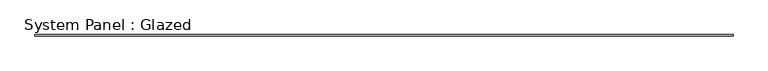
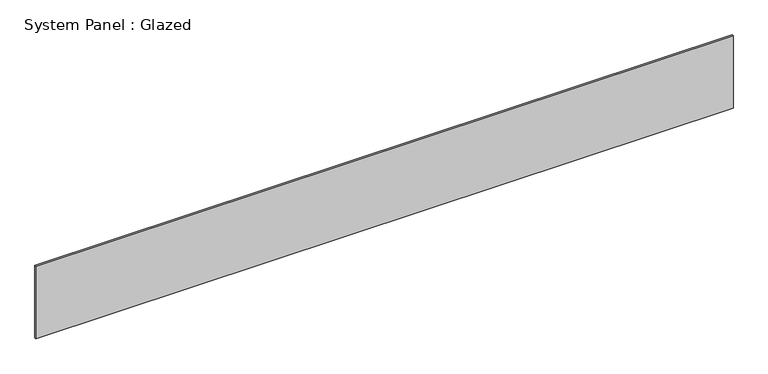
"""IFC4 building model written with IfcOpenShell, lengths in millimetres: plate geometry, System Panel : Glazed."""

from ifc_helpers import new_model, si_unit, origin, origin_with_axes, place, context, project, spatial, polyline, outline, extrude, source, transform, mapped, element, save


def system_panel_glazed_48350550(model_context):
    return source(origin(), model_context, "Body", "SweptSolid", [
        extrude(outline(polyline([(6934.2, 19.05), (-6934.2, 19.05), (-6934.2, 44.45), (6934.2, 44.45), (6934.2, 19.05)])), origin_with_axes(), (0.0, 0.0, 1.0), 1524.0),
    ])


if __name__ == "__main__":
    model = new_model("IFC4")
    model_context = context("Model", 3, world=origin())
    ifc_project = project(units=[si_unit("LENGTHUNIT", "METRE", prefix="MILLI")], contexts=[model_context])
    site = spatial("IfcSite", under=ifc_project)
    building = spatial("IfcBuilding", under=site)
    placement = place(None, origin())
    system_panel_glazed_shape = system_panel_glazed_48350550(model_context)
    element("IfcPlate", 1, ObjectType="System Panel : Glazed", at=placement, inside=building, context=model_context, shape_type="MappedRepresentation", body=[
        mapped(system_panel_glazed_shape, transform((0.0, 0.0, 0.0), x_axis=(1.0, 0.0, 0.0), y_axis=(0.0, 1.0, 0.0), z_axis=(0.0, 0.0, 1.0))),
    ])
    save(model, "model.ifc")

# Revit data of these elements
# Type "System Panel : Glazed"
#   Construction Type Id = "GSP4R"
#   Analytic Construction = "1/8 in Pilkington single glazing"
#   Visual Light Transmittance = 0.9
#   Solar Heat Gain Coefficient = 0.86
#   Heat Transfer Coefficient (U) = 1.18115 BTU/(h·ft²·°F)
# Element 1 (IfcPlate, "System Panel : Glazed")
#   Materials on its faces: "Glass"
# Materials
#   "Glass": class "Glass", colour RGB 0 128 192, transparency 0.75, Description = "Soda Lime Glass", Cost = 0
